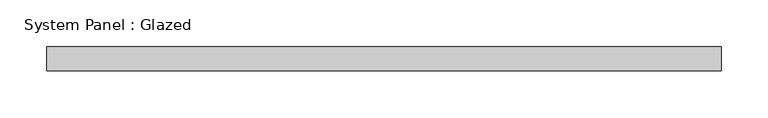
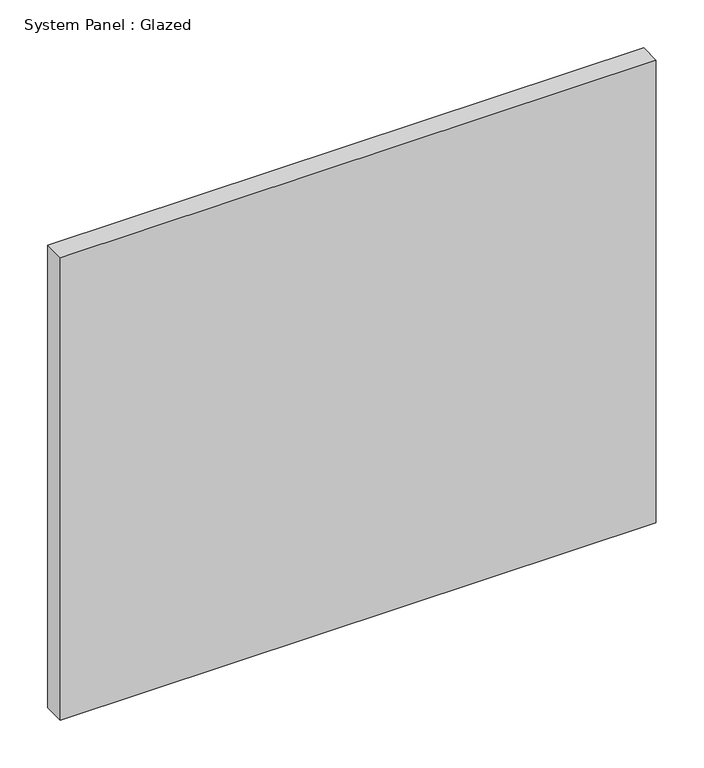
"""IFC4 building model written with IfcOpenShell, lengths in millimetres: plate geometry, System Panel : Glazed."""

from ifc_helpers import new_model, si_unit, origin, origin_with_axes, place, context, project, spatial, polyline, outline, extrude, source, transform, mapped, element, save


def system_panel_glazed_17d59646(model_context):
    return source(origin(), model_context, "Body", "SweptSolid", [
        extrude(outline(polyline([(358.775, 19.05), (-358.775, 19.05), (-358.775, 44.45), (358.775, 44.45), (358.775, 19.05)])), origin_with_axes(), (0.0, 0.0, 1.0), 588.4067525),
    ])


if __name__ == "__main__":
    model = new_model("IFC4")
    model_context = context("Model", 3, world=origin())
    ifc_project = project(units=[si_unit("LENGTHUNIT", "METRE", prefix="MILLI")], contexts=[model_context])
    site = spatial("IfcSite", under=ifc_project)
    building = spatial("IfcBuilding", under=site)
    placement = place(None, origin())
    system_panel_glazed_shape = system_panel_glazed_17d59646(model_context)
    element("IfcPlate", 1, ObjectType="System Panel : Glazed", at=placement, inside=building, context=model_context, shape_type="MappedRepresentation", body=[
        mapped(system_panel_glazed_shape, transform((0.0, 0.0, 0.0), x_axis=(1.0, 0.0, 0.0), y_axis=(0.0, 1.0, 0.0), z_axis=(0.0, 0.0, 1.0))),
    ])
    save(model, "model.ifc")

# Revit data of these elements
# Type "System Panel : Glazed"
#   Construction Type Id = "GSP4R"
#   Analytic Construction = "1/8 in Pilkington single glazing"
#   Visual Light Transmittance = 0.9
#   Solar Heat Gain Coefficient = 0.86
#   Heat Transfer Coefficient (U) = 1.18115 BTU/(h·ft²·°F)
#   Define Thermal Properties by = 1
# Element 1 (IfcPlate, "System Panel : Glazed")
#   Materials on its faces: "Glass"
# Materials
#   "Glass": class "Glass", colour RGB 0 128 192, transparency 0.75, Description = "Soda Lime Glass", Cost = 0
